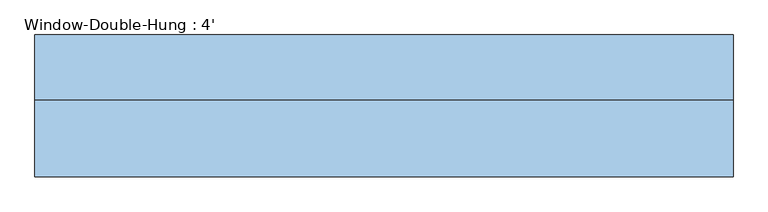
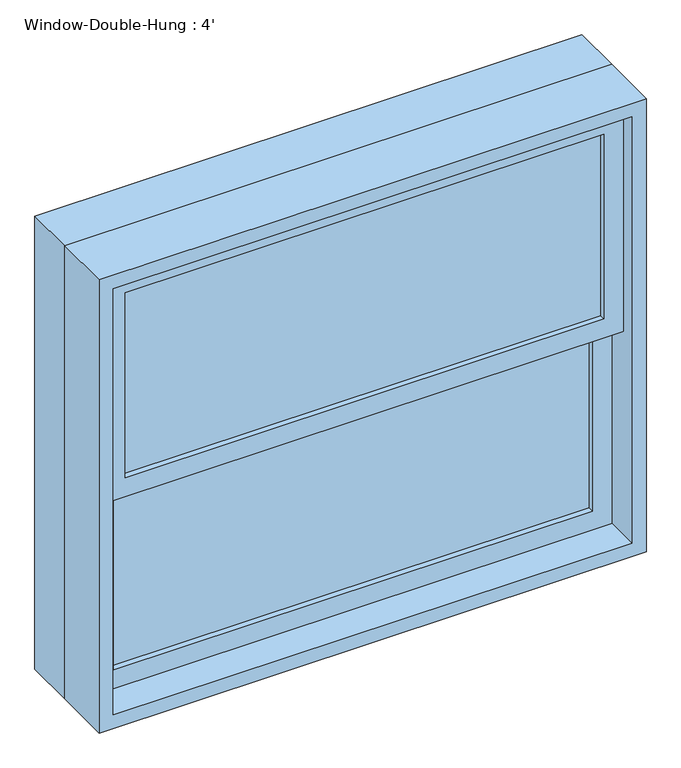
"""IFC4 building model written with IfcOpenShell, lengths in millimetres: window geometry, Window-Double-Hung : 4'."""

from ifc_helpers import new_model, si_unit, frame, origin, place, context, project, spatial, polyline, outline, extrude, source, transform, mapped, element, save


def window_double_hung_4_aab3aae7(model_context):
    return source(origin(), model_context, "Body", "SweptSolid", [
        extrude(outline(polyline([(533.4, -44.45), (-533.4, -44.45), (-533.4, -38.1), (533.4, -38.1), (533.4, -44.45)])), frame((0.0, 0.0, 990.6), z_axis=(0.0, 0.0, 1.0), x_axis=(1.0, 0.0, 0.0)), (0.0, 0.0, 1.0), 434.975),
        extrude(outline(polyline([(-533.4, -31.75), (-533.4, -25.4), (533.4, -25.4), (533.4, -31.75), (-533.4, -31.75)])), frame((0.0, 0.0, 990.6), z_axis=(0.0, 0.0, 1.0), x_axis=(1.0, 0.0, 0.0)), (0.0, 0.0, 1.0), 434.975),
        extrude(outline(polyline([(533.4, -88.9), (-533.4, -88.9), (-533.4, -82.55), (533.4, -82.55), (533.4, -88.9)])), frame((0.0, 0.0, 1470.025), z_axis=(0.0, 0.0, 1.0), x_axis=(1.0, 0.0, 0.0)), (0.0, 0.0, 1.0), 434.975),
        extrude(outline(polyline([(-533.4, -76.2), (-533.4, -69.85), (533.4, -69.85), (533.4, -76.2), (-533.4, -76.2)])), frame((0.0, 0.0, 1470.025), z_axis=(0.0, 0.0, 1.0), x_axis=(1.0, 0.0, 0.0)), (0.0, 0.0, 1.0), 434.975),
        extrude(outline(polyline([(1470.025, 577.85), (1470.025, -577.85), (946.15, -577.85), (946.15, 577.85), (1470.025, 577.85)]), holes=[polyline([(1425.575, -533.4), (1425.575, 533.4), (990.6, 533.4), (990.6, -533.4), (1425.575, -533.4)])]), frame((0.0, -57.15, 0.0), z_axis=(0.0, 1.0, 0.0), x_axis=(0.0, 0.0, 1.0)), (0.0, 0.0, 1.0), 44.45),
        extrude(outline(polyline([(1949.45, 577.85), (1949.45, -577.85), (1425.575, -577.85), (1425.575, 577.85), (1949.45, 577.85)]), holes=[polyline([(1905.0, -533.4), (1905.0, 533.4), (1470.025, 533.4), (1470.025, -533.4), (1905.0, -533.4)])]), frame((0.0, -101.6, 0.0), z_axis=(0.0, 1.0, 0.0), x_axis=(0.0, 0.0, 1.0)), (0.0, 0.0, 1.0), 44.45),
        extrude(outline(polyline([(1981.2, 609.6), (1981.2, -609.6), (914.4, -609.6), (914.4, 609.6), (1981.2, 609.6)]), holes=[polyline([(1949.45, -577.85), (1949.45, 577.85), (946.15, 577.85), (946.15, -577.85), (1949.45, -577.85)])]), frame((0.0, -133.35, 0.0), z_axis=(0.0, 1.0, 0.0), x_axis=(0.0, 0.0, 1.0)), (0.0, 0.0, 1.0), 133.35),
        extrude(outline(polyline([(1981.2, 609.6), (1981.2, -609.6), (914.4, -609.6), (914.4, 609.6), (1981.2, 609.6)]), holes=[polyline([(1962.15, 590.55), (933.45, 590.55), (933.45, -590.55), (1962.15, -590.55), (1962.15, 590.55)])]), frame((0.0, 0.0, 0.0), z_axis=(0.0, 1.0, 0.0), x_axis=(0.0, 0.0, 1.0)), (0.0, 0.0, 1.0), 114.3),
    ])


if __name__ == "__main__":
    model = new_model("IFC4")
    model_context = context("Model", 3, world=origin())
    ifc_project = project(units=[si_unit("LENGTHUNIT", "METRE", prefix="MILLI")], contexts=[model_context])
    site = spatial("IfcSite", under=ifc_project)
    building = spatial("IfcBuilding", under=site)
    placement = place(None, origin())
    window_double_hung_4_shape = window_double_hung_4_aab3aae7(model_context)
    element("IfcWindow", 1, ObjectType="Window-Double-Hung : 4'", at=placement, inside=building, context=model_context, shape_type="MappedRepresentation", body=[
        mapped(window_double_hung_4_shape, transform((0.0, 0.0, 0.0), x_axis=(1.0, 0.0, 0.0), y_axis=(0.0, 1.0, 0.0), z_axis=(0.0, 0.0, 1.0))),
    ])
    save(model, "model.ifc")

# Revit data of these elements
# Type "Window-Double-Hung : 4'"
#   Type Mark = "18"
#   Fire Rating = "0.5h"
#   Construction Type Id = "DG-DR"
#   Assembly Code = "B2020100"
#   Analytic Construction = "Double glazing - domestic"
#   Wall Thickness [instance default] = 0' - 6"
#   Window Inset [instance default] = 0' - 0"
#   Visual Light Transmittance = 0.81
#   Thermal Resistance (R) = 1.8146 (h·ft²·°F)/BTU
#   Solar Heat Gain Coefficient = 0.76
#   Muntin Width = 3' - 6"
#   Muntin Height = 1' - 5 1/8"
#   Interior Wall Closure [instance default] = 0' - 1 1/2"
#   Rough Width = 4' - 0 1/2"
#   Rough Height = 3' - 6 1/2"
#   Frame Extension [instance default] = 0' - 1 1/4"
#   Exterior Wall Closure [instance default] = 0' - 0 1/2"
#   Extension Jamb [instance default] = 0' - 1 1/2"
#   Heat Transfer Coefficient (U) = 0.5511 BTU/(h·ft²·°F)
#   Height = 3' - 6"
#   Width = 4' - 0"
#   Top Muntin Visibility = yes
#   Indicator Visibility [instance default] = yes
#   Extension Jamb Visibility [instance default] = yes
#   Interior Trim Visibility [instance default] = yes
#   Exterior Trim Visibility [instance default] = yes
#   Define Thermal Properties by = 1
#   Bottom Muntin Visibility = yes
#   Muntin Pattern = Muntin Pattern_2x2 : Muntin Pattern_2x2
#   Interior Trim Material = Wood - Stained
#   Interior Trim = Trim-Window-Interior-Flat : Picture Frame
#   Exterior Trim Material = Clad - White
#   Exterior Trim = Trim-Window-Exterior-Flat : with Sill
#   Glass Panel Material = Glass
#   Exterior Frame Material = Clad - White
#   Interior Frame Material = Wood - Stained
#   Wall Closure = (empty or 0)
# Element 1 (IfcWindow, "Window-Double-Hung : 4'")
#   Wall Thickness = 0' - 9"
#   Extension Jamb = 0' - 4 1/2"
#   Materials on its faces: "Wood - Stained", "Glass", "Clad - White"
# Materials
#   "Wood - Stained": class "Wood", colour RGB 224 178 126, transparency 0, Cost = 0
#   "Clad - White": class "Wood", colour RGB 242 242 238, transparency 0, Cost = 0
#   "Glass": class "Glass", colour RGB 0 128 192, transparency 0.75, Description = "Soda Lime Glass", Cost = 0
